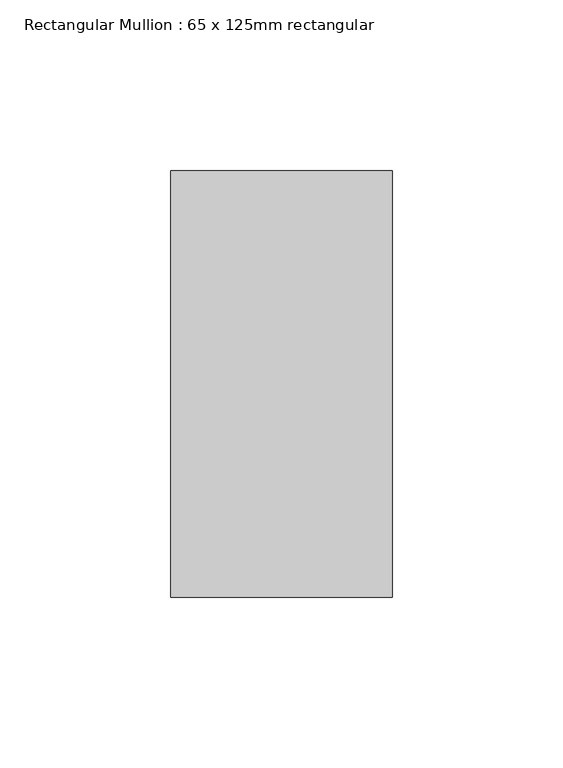
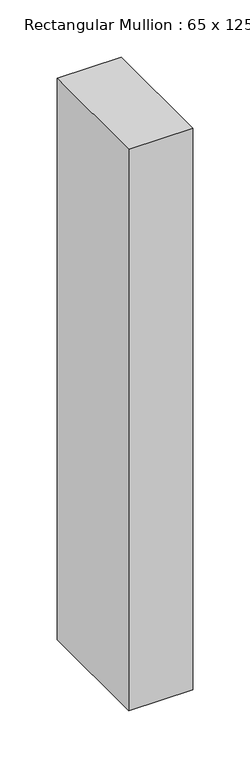
"""IFC4 building model written with IfcOpenShell, lengths in millimetres: member geometry, Rectangular Mullion : 65 x 125mm rectangular."""

from ifc_helpers import new_model, si_unit, frame, origin, place, context, project, spatial, polyline, outline, extrude, source, transform, mapped, element, save


def rectangular_mullion_65_x_125mm_rectangular_e22a5c8f(model_context):
    return source(origin(), model_context, "Body", "SweptSolid", [
        extrude(outline(polyline([(0.0, 62.5), (0.0, -62.5), (-65.0, -62.5), (-65.0, 62.5), (0.0, 62.5)])), frame((0.0, 0.0, -600.0), z_axis=(0.0, 0.0, 1.0), x_axis=(1.0, 0.0, 0.0)), (0.0, 0.0, 1.0), 600.0),
    ])


if __name__ == "__main__":
    model = new_model("IFC4")
    model_context = context("Model", 3, world=origin())
    ifc_project = project(units=[si_unit("LENGTHUNIT", "METRE", prefix="MILLI")], contexts=[model_context])
    site = spatial("IfcSite", under=ifc_project)
    building = spatial("IfcBuilding", under=site)
    placement = place(None, origin())
    rectangular_mullion_65_x_125mm_rectangular_shape = rectangular_mullion_65_x_125mm_rectangular_e22a5c8f(model_context)
    element("IfcMember", 1, ObjectType="Rectangular Mullion : 65 x 125mm rectangular", at=placement, inside=building, context=model_context, shape_type="MappedRepresentation", body=[
        mapped(rectangular_mullion_65_x_125mm_rectangular_shape, transform((0.0, 0.0, 0.0), x_axis=(1.0, 0.0, 0.0), y_axis=(0.0, 1.0, 0.0), z_axis=(0.0, 0.0, 1.0))),
    ])
    save(model, "model.ifc")

# Revit data of these elements
# Type "Rectangular Mullion : 65 x 125mm rectangular"
#   built-in parameter 1007304 = 0.410105 (stored number, unit not read)
#   built-in parameter 1007301 = 0.106627 (stored number, unit not read)
#   built-in parameter 1007300 = 0.106627 (stored number, unit not read)
# Element 1 (IfcMember, "Rectangular Mullion : 65 x 125mm rectangular")
#   Materials on its faces: "Aluminum"
# Materials
#   "Aluminum": class "Metal", colour RGB 244 245 246, transparency 0, Description = "Aluminum 6061", Cost = 0
